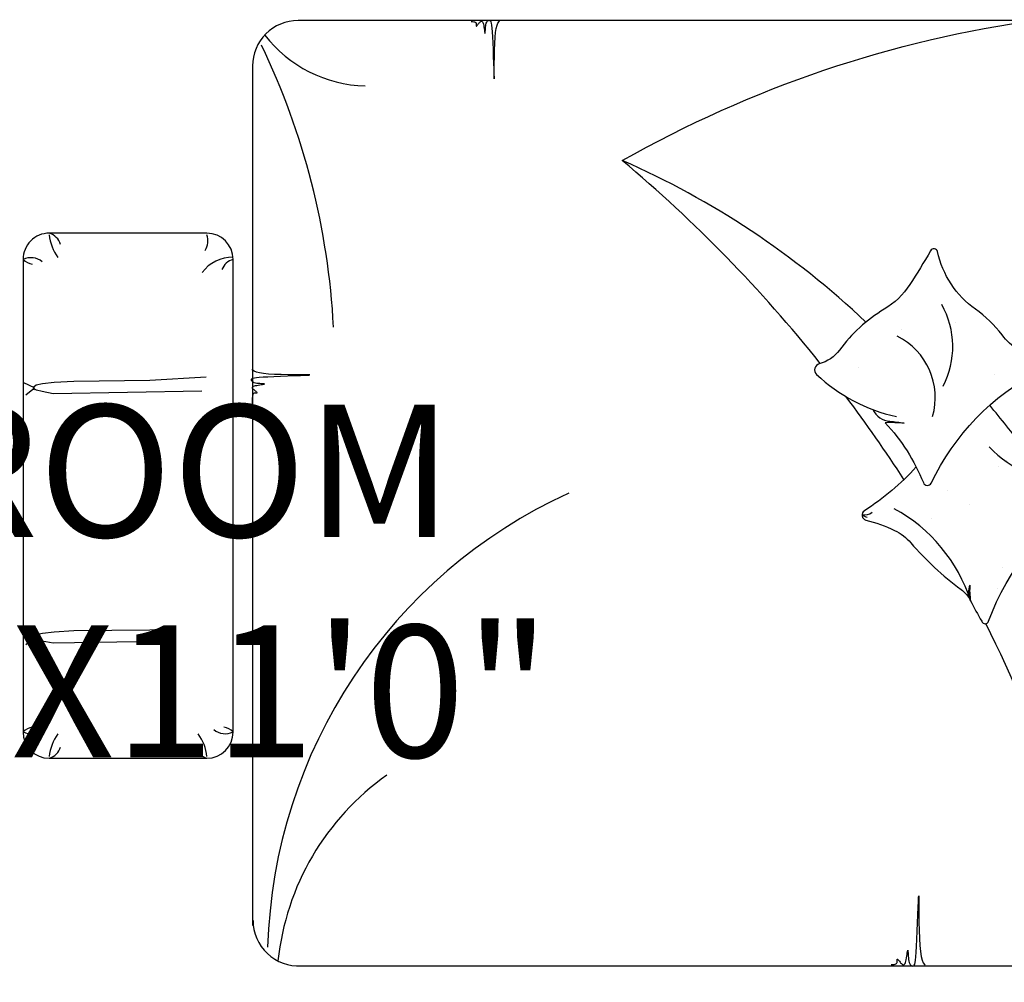
# Model space of a CAD drawing. Units: inches. Extents: x 3592 to 4861, y 1650 to 2243.
# Tile 15 of 30: x 4306 to 4365, y 1812 to 1870. Entities that reach past the tile are written whole.
import ezdxf

# ---------------------------------------------------------------- set-up
doc = ezdxf.new("R2010")
doc.units = ezdxf.units.IN
for name, color, linetype, lineweight in [('A-ANNO-DIMS', 2, 'Continuous', 13), ('A-AREA-IDEN', 7, 'Continuous', 18), ('A-FURN', 9, 'Continuous', 13)]:
    doc.layers.add(name, color=color, linetype=linetype, lineweight=lineweight)
doc.layers.add('FUR', color=42, linetype='Continuous')
doc.styles.get("Standard").update_dxf_attribs({"font": 'arial.ttf'})
doc.dimstyles.new('ISO-25', dxfattribs={"dimtxt": 9, "dimasz": 2.5, "dimexe": 1.25, "dimexo": 0.625, "dimtad": 1, "dimlunit": 3, "dimtxsty": 'Standard', "dimcen": 2.5, "dimadec": 0, "dimazin": 0, "dimtfac": 1, "dimtmove": 0, "dimatfit": 3, "dimfxl": 1, "dimarcsym": 0})

# ---------------------------------------------------------------- blocks, each defined once
blk = doc.blocks.new('*X20')
at = {"color": 0}
for p, q in [((3155.9, 8182.9), (3155.9, 8182.9)), ((3147.8, 8143.4), (3147.8, 8143.4)), ((3283, 8049.6), (3283, 8049.6)), ((3209.5, 8023.9), (3209.5, 8023.9)), ((3251.6, 7997), (3251.6, 7997)), ((3154.1, 7950.7), (3154.1, 7950.7))]:
    blk.add_line(p, q, dxfattribs=at)
blk = doc.blocks.new('*X19')
at = {"color": 0}
for p, q in [((3155.9, 8182.9), (3155.9, 8182.9)), ((3139.8, 7939.7), (3139.8, 7939.7))]:
    blk.add_line(p, q, dxfattribs=at)
blk = doc.blocks.new('*X18')
at = {"color": 0}
for p, q in [((3155.9, 8182.9), (3155.9, 8182.9)), ((3139.8, 7939.7), (3139.8, 7939.7))]:
    blk.add_line(p, q, dxfattribs=at)
blk = doc.blocks.new('*X17')
at = {"color": 0}
for p, q in [((3163, 7776.2), (3163, 7776.2)), ((3422.2, 7761.3), (3422.2, 7761.3)), ((3244.3, 7698.6), (3244.3, 7698.6)), ((3340.3, 7689.4), (3340.3, 7689.4)), ((3236.2, 7675.7), (3236.2, 7675.7))]:
    blk.add_line(p, q, dxfattribs=at)
blk = doc.blocks.new('BED1')
for p, q in [((2058.7, 800), (150, 800)), ((2537.2, 404.9), (2237.2, 404.9)), ((2187.2, 354.9), (2187.2, -545.1)), ((2587.2, -545.1), (2587.2, 354.9)), ((2582, 188.1), (2565.4, 174.8)), ((2566.3, 178.5), (2565.2, 177.4)), ((2565.4, 174.8), (2585.7, 165.4)), ((2566.3, -296.8), (2565.2, -297.9)), ((2582, -287.1), (2565.4, -300.5)), ((2565.4, -300.5), (2585.7, -309.9)), ((2237.2, -595.1), (2537.2, -595.1)), ((150, -1000), (2063.5, -1000))]:
    blk.add_line(p, q)
for points in [[(934, 797.9), (930.9, 797.7), (928.3, 797.4), (926.3, 796.9), (924.9, 796.3), (923.8, 795.6), (923.1, 794.8), (922.7, 793.8), (922.5, 792.7), (922.4, 791.5), (922.5, 790.3), (922.6, 789.2), (922.6, 788.3), (922.6, 787.6), (922.4, 787.3), (922, 787.4), (921.4, 787.9), (920.6, 788.9), (919.5, 790.2), (918.4, 791.6), (917.1, 793.1), (915.9, 794.6), (914.6, 796), (913.3, 797.1), (912.2, 797.9), (911.1, 798.3), (910.1, 798.4), (909.2, 798), (908.3, 797.1), (907.5, 795.8), (906.8, 793.9), (906, 791.4), (905.4, 788.5), (904.8, 785.2), (904.2, 781.7), (903.7, 778.4), (903.2, 775.4), (902.8, 772.9), (902.5, 771.3), (902.3, 770.6), (902.1, 771.2), (902, 772.8), (901.8, 775.2), (901.7, 778.1), (901.5, 781.5), (901.2, 785), (900.8, 788.4), (900.2, 791.5), (899.5, 794.1), (898.6, 796.2), (897.6, 797.9), (896.5, 799.2), (895.3, 800), (894.1, 800.5), (893, 800.7), (891.9, 800.5), (890.9, 800.1), (890, 799), (889.1, 797.1), (888.3, 794), (887.6, 789.3), (886.9, 782.9), (886.2, 774.2), (885.5, 763.1), (884.8, 749.5), (884.2, 734.2), (883.6, 718.3), (883, 702.8), (882.5, 688.8), (882, 677.5), (881.7, 669.8), (881.5, 666.9), (881.3, 669.4), (881.3, 676.7), (881.3, 687.8), (881.2, 701.5), (881.1, 716.8), (880.8, 732.6), (880.2, 748), (879.4, 761.8), (878.3, 773.2), (876.9, 782.2), (875.1, 789.2), (872.9, 794.4), (870.3, 798), (869, 799)], [(2150, -913.5), (2150, 723.2)], [(2327.6, 182.3), (2530, 185.9), (2550.8, 181.9), (2561.7, 179), (2566, 176.7), (2566.9, 174.4), (2566.3, 171.9), (2562, 169.2), (2550.3, 166.5), (2527.7, 163.9), (2490.6, 161.8), (2345.5, 160.2), (2317.8, 158.5)], [(2149.7, -259.9), (2150, -268.4), (2150.1, -274.1), (2150.1, -278.1), (2150, -281.4), (2149.8, -284), (2149.5, -286.1), (2149.1, -287.8), (2148.7, -289), (2148.1, -289.9), (2147.4, -290.5), (2146.6, -290.8), (2145.6, -291), (2144.6, -291), (2143.6, -291), (2142.7, -290.9), (2141.9, -290.9), (2141.4, -290.9), (2141.1, -291), (2141.2, -291.4), (2141.7, -291.9), (2142.5, -292.6), (2143.5, -293.4), (2144.7, -294.4), (2146, -295.4), (2147.2, -296.5), (2148.4, -297.6), (2149.3, -298.6), (2150, -299.6), (2150.3, -300.5), (2150.4, -301.3), (2150, -302.1), (2149.3, -302.8), (2148.2, -303.5), (2146.6, -304.1), (2144.6, -304.7), (2142.1, -305.2), (2139.3, -305.7), (2136.5, -306.2), (2133.7, -306.6), (2131.2, -307), (2129.2, -307.3), (2127.8, -307.6), (2127.3, -307.8), (2127.7, -308), (2129, -308.1), (2131, -308.2), (2133.5, -308.3), (2136.3, -308.5), (2139.2, -308.7), (2142, -309), (2144.6, -309.5), (2146.8, -310.1), (2148.6, -310.9), (2150, -311.7), (2151, -312.7), (2151.7, -313.6), (2152.1, -314.6), (2152.3, -315.6), (2152.2, -316.5), (2151.8, -317.3), (2150.9, -318.1), (2149.3, -318.8), (2146.7, -319.4), (2142.8, -320), (2137.4, -320.6), (2130.2, -321.2), (2121, -321.8), (2109.7, -322.3), (2096.9, -322.9), (2083.6, -323.4), (2070.7, -323.9), (2059.1, -324.3), (2049.6, -324.7), (2043.2, -325), (2040.8, -325.2), (2042.9, -325.3), (2049, -325.3), (2058.2, -325.3), (2069.6, -325.4), (2082.3, -325.5), (2095.6, -325.8), (2108.4, -326.2), (2119.9, -326.8), (2129.4, -327.8), (2136.9, -329), (2142.7, -330.5), (2147, -332.3), (2150, -334.4), (2150.9, -335.6)], [(2246.5, -294.4), (2530, -289.4), (2550.8, -293.4), (2561.7, -296.3), (2566, -298.6), (2566.9, -300.8), (2566.3, -303.4), (2562, -306.1), (2550.3, -308.8), (2527.7, -311.3), (2490.6, -313.5), (2345.5, -315), (2238.6, -321.8)], [(1733.7, -998.3), (1731.1, -998.1), (1729, -997.8), (1727.4, -997.4), (1726.1, -997), (1725.2, -996.4), (1724.7, -995.7), (1724.3, -994.8), (1724.1, -993.9), (1724.1, -992.9), (1724.1, -991.9), (1724.2, -991), (1724.2, -990.2), (1724.2, -989.7), (1724.1, -989.4), (1723.8, -989.5), (1723.2, -990), (1722.5, -990.8), (1721.7, -991.8), (1720.7, -993), (1719.7, -994.3), (1718.6, -995.5), (1717.5, -996.6), (1716.5, -997.6), (1715.5, -998.3), (1714.6, -998.6), (1713.8, -998.6), (1713, -998.3), (1712.3, -997.6), (1711.7, -996.5), (1711, -994.9), (1710.4, -992.9), (1709.9, -990.4), (1709.4, -987.6), (1708.9, -984.8), (1708.5, -982), (1708.1, -979.5), (1707.8, -977.4), (1707.5, -976.1), (1707.3, -975.5), (1707.1, -976), (1707, -977.3), (1706.9, -979.3), (1706.8, -981.8), (1706.7, -984.6), (1706.4, -987.5), (1706.1, -990.3), (1705.6, -992.9), (1705, -995.1), (1704.2, -996.9), (1703.4, -998.3), (1702.4, -999.3), (1701.5, -1000), (1700.5, -1000.4), (1699.6, -1000.6), (1698.7, -1000.4), (1697.8, -1000.1), (1697, -999.2), (1696.3, -997.6), (1695.7, -995), (1695.1, -991.1), (1694.5, -985.7), (1693.9, -978.5), (1693.3, -969.3), (1692.8, -957.9), (1692.2, -945.2), (1691.7, -931.9), (1691.2, -919), (1690.8, -907.4), (1690.4, -897.9), (1690.1, -891.5), (1689.9, -889.1), (1689.8, -891.2), (1689.8, -897.3), (1689.8, -906.5), (1689.7, -917.9), (1689.6, -930.6), (1689.4, -943.8), (1688.9, -956.6), (1688.3, -968.1), (1687.3, -977.6), (1686.1, -985.2), (1684.6, -991), (1682.8, -995.3), (1680.7, -998.3), (1679.6, -999.2)]]:
    blk.add_lwpolyline(points)
for points in [[(886.4, -150, -0.069098), (985, -66.5, 0.658965), (982.1, -48.7, -0.049789), (927.4, -29, -0.103757), (896.6, -5.4, 0.055725), (800.9, 83.3, -0.11866), (782.7, 104.9, 0.016811), (761.6, 143.9, 0.70791), (748.3, 144, -0.16964), (551.9, -96.6, 0.664036), (554, -110.7, 0.023706), (627, -144.7, -0.134834), (683.2, -188, 0.012748), (746.3, -267.4)], [(969.1, -259.1, 0.263265), (936.3, -236.9, -0.026108), (909.2, -233.2, 0.027613), (945.1, -234.2, -0.089259), (872.7, -120, 0.662242), (857.6, -119.3, -0.162037), (651.8, -332.7, 0.676499), (654, -354.5, -0.160513), (722.9, -401.5, 0.07473), (773.5, -450.3, -0.187721), (845.5, -559.9, 0.70791), (858.8, -561.4, -0.010003), (898.6, -497.3, -0.113819), (947.3, -450.2, 0.099539), (1032.5, -372.4, -0.173425), (1070.9, -346.4, 0.589988), (1076.2, -326.1, 0.137312), (923.9, -245.9, 0.137312)], [(1446, -733.4, -0.095039), (652.8, -1001.7)]]:
    blk.add_lwpolyline(points, format="xyb")
for centre, radius, start, end in [((3208.8, 1363.3), 2739.4, 191.8679, 206.3247), ((1608.1, 842.5), 496.3, 305.1901, 354.0206), ((2062.7, 713.7), 86.5, 0, 93.5376), ((1138.6, 793.9), 983.2, 294.6078, 358.3033), ((2237.2, 354.9), 50, 90, 180), ((2321.1, 409.7), 84.5, 185.6196, 217.1396), ((2227.5, 373.5), 32.8, 17.833, 72.8005), ((2546.9, 373.5), 32.8, 107.1995, 162.167), ((2453.3, 409.7), 84.5, 322.8604, 354.3804), ((2537.2, 354.9), 50, 0, 90), ((2201.9, 323.3), 34.8, 50.8413, 114.9586), ((2572.5, 323.3), 34.8, 65.0414, 129.1587), ((2212.2, 381.5), 36.5, 226.8095, 258.3841), ((2562.2, 381.5), 36.5, 281.6159, 313.1905), ((751.8, 88.7), 34.9, 336.8352, 27.7218), ((684.2, 86), 100.3, 353.675, 10.882), ((1074.1, 198.8), 306.1, 197.8602, 241.5122), ((978.5, -68.6), 14.3, 39.7097, 85.9506), ((983.7, -79.5), 20.8, 73.7967, 130.4566), ((602.5, -324), 198.6, 43.2035, 95.0556), ((3208.8, 1363.3), 2739.4, 212.9314, 216.951), ((981.1, -281.8), 131.1, 164.0372, 243.4536), ((980, -379), 163.4, 152.6104, 209.361), ((3208.8, 1363.3), 2739.4, 218.6329, 229.9449), ((2098.7, 754.7), 1625, 226.5887, 246.3156), ((3402.5, -342.9), 1408.5, 182.9917, 205.6819), ((2188.1, -476.2), 73, 269.4513, 322.8027), ((2178, -513.5), 33, 286.1827, 338.1386), ((2572.5, -513.6), 34.8, 230.8413, 294.9586), ((2562.2, -571.8), 36.5, 46.8095, 78.3841), ((2237.2, -545.1), 50, 180, 270), ((2271.1, -580.9), 35.8, 148.9055, 197.5541), ((2453.3, -600), 84.5, 5.6196, 37.1396), ((2537.2, -545.1), 50, 270, 0), ((2546.9, -563.8), 32.8, 197.833, 252.8005), ((1929.1, -1126), 250.5, 37.8553, 88.4405), ((2063.5, -913.5), 86.5, 270, 0)]:
    blk.add_arc(centre, radius, start, end)
for name in ['*X19', '*X18', '*X20', '*X17']:
    blk.add_blockref(name, (-2425.3, -8101.4))
blk = doc.blocks.new('A$C68AE1801')
at = {"layer": 'FUR', "xscale": 0.001, "yscale": 0.001, "zscale": 0.001, "rotation": 180}
blk.add_blockref('BED1', (2.5872, 1.49), dxfattribs=at)
blk = doc.blocks.new('*D156')
at = {"layer": 'A-ANNO-DIMS', "color": 0, "lineweight": -2, "transparency": 16777216}
for p, q in [((4291.393, 1793.561), (4291.393, 1804.979)), ((4363.347, 1793.561), (4363.347, 1804.979)), ((4291.393, 1803.729), (4155.277, 1803.729)), ((4360.847, 1803.729), (4293.893, 1803.729))]:
    blk.add_line(p, q, dxfattribs=at)
at = {"layer": 'A-ANNO-DIMS', "color": 0, "transparency": 16777216}
for points in [[(4293.893, 1804.145), (4293.893, 1803.312), (4291.393, 1803.729)], [(4360.847, 1804.145), (4360.847, 1803.312), (4363.347, 1803.729)]]:
    blk.add_solid(points, dxfattribs=at)
at = {"layer": 'Defpoints', "color": 0, "transparency": 16777216}
for p in [(4291.393, 1803.729), (4291.393, 1792.936), (4363.347, 1792.936)]:
    blk.add_point(p, dxfattribs=at)
at = {"layer": 'A-ANNO-DIMS', "color": 0, "transparency": 16777216, "insert": (4222.085, 1809.01), "char_height": 9, "attachment_point": 5}
blk.add_mtext('SIDEBOARD 6\'-0" TYP.', dxfattribs=at)

msp = doc.modelspace()

# ---------------------------------------------------------------- block references
at = {"layer": 'A-FURN', "xscale": 31.7658940618111, "yscale": 31.7658940618111, "zscale": 31.7658940618111}
msp.add_blockref('A$C68AE1801', (4305.708, 1790.711), dxfattribs=at)

# ---------------------------------------------------------------- texts
at = {"layer": 'A-AREA-IDEN', "insert": (4278.607, 1846.565), "char_height": 8, "attachment_point": 1}
msp.add_mtext_dynamic_manual_height_columns('BEDROOM\\P10\'4"X11\'0"', width=121.44943, gutter_width=12.5, heights=[0], dxfattribs=at)

# ---------------------------------------------------------------- dimensions: what is measured, and where the dimension line sits
at = {"layer": 'A-ANNO-DIMS'}
dim = msp.add_linear_dim(base=(4291.393, 1803.729), p1=(4363.347, 1792.936), p2=(4291.393, 1792.936), angle=180, text='SIDEBOARD <> TYP.', dimstyle='ISO-25', override={"dimdec": 1, "dimlfac": 1, "dimrnd": 0, "dimzin": 1, "dimdsep": 46, "dimlunit": 4, "dimfrac": 2}, dxfattribs=at)
dim.commit()
dim.dimension.update_dxf_attribs({"geometry": '*D156', "text_midpoint": (4222.085, 1809.01)})

doc.saveas('drawing.dxf')
